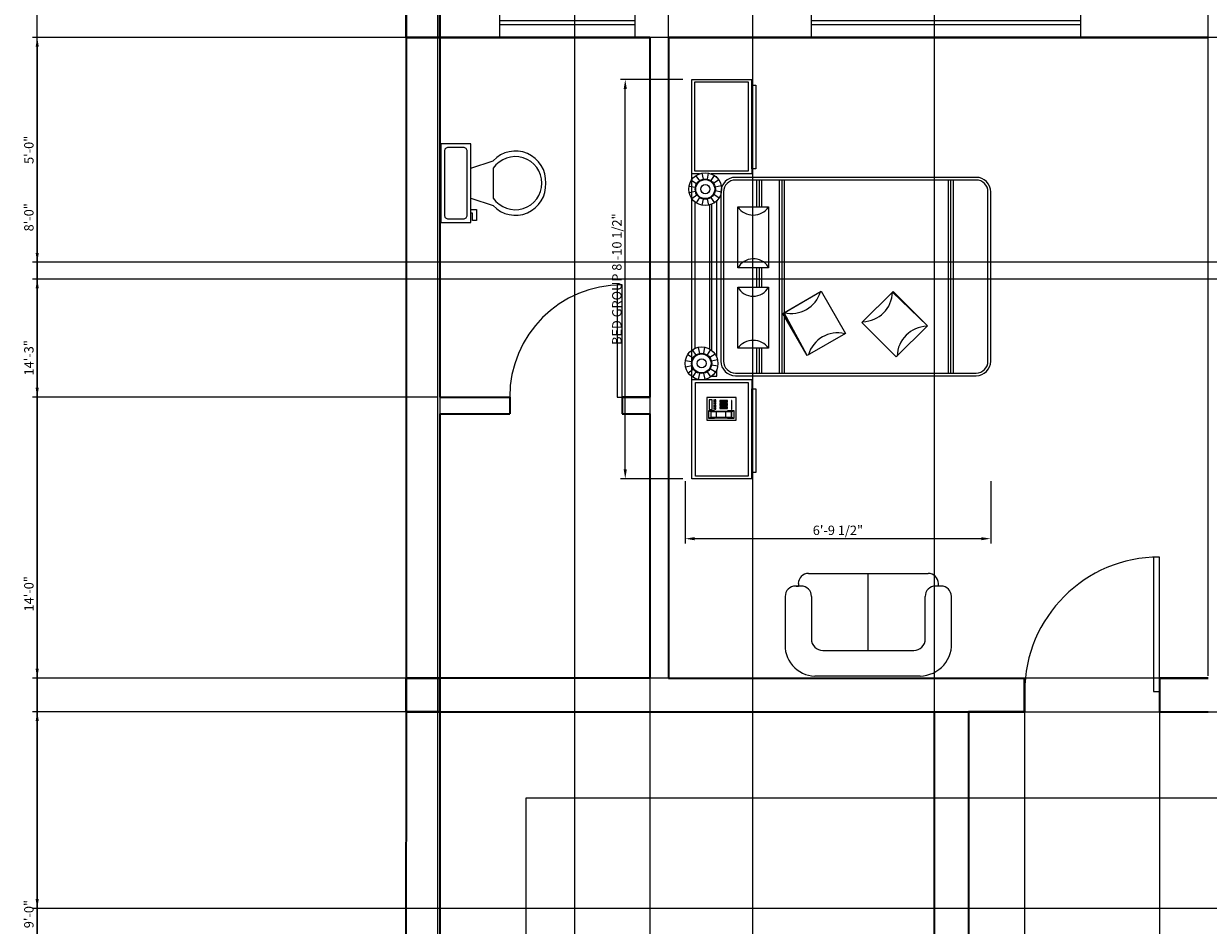
# Model space of a CAD drawing. Units: inches. Extents: x 1624 to 3956, y 1589 to 5028.
# Tile 9 of 16: x 1627 to 1943, y 2250 to 2490. Entities that reach past the tile are written whole.
import ezdxf

# ---------------------------------------------------------------- set-up
doc = ezdxf.new("R2010")
doc.units = ezdxf.units.IN
for name, color, linetype, lineweight in [('A-ANNO-DIMS', 2, 'Continuous', 13), ('A-COLS', 1, 'Continuous', 40), ('A-DOOR', 3, 'Continuous', 18), ('A-FLOR-CASE', 32, 'Continuous', 25), ('A-FLOR-FIXT', 9, 'Continuous', 18), ('A-FURN', 8, 'Continuous', 18), ('A-GLAZ', 4, 'Continuous', 18), ('A-WALL', 7, 'Continuous', 35)]:
    doc.layers.add(name, color=color, linetype=linetype, lineweight=lineweight)
doc.styles.get("Standard").update_dxf_attribs({"font": 'arial.ttf'})
doc.dimstyles.new('Copy of ISO-25', dxfattribs={"dimtxt": 2.5, "dimasz": 2.5, "dimexe": 1.25, "dimexo": 0.625, "dimtad": 1, "dimdec": 1, "dimlunit": 4, "dimtxsty": 'Standard', "dimcen": 2.5, "dimadec": 0, "dimazin": 0, "dimtfac": 1, "dimtdec": 1, "dimtmove": 0, "dimatfit": 3, "dimfxl": 1, "dimarcsym": 0})

# ---------------------------------------------------------------- blocks, each defined once
blk = doc.blocks.new('*U4')
for p, q in [((0, 0), (0, -6)), ((-40, 0), (-40, -6))]:
    blk.add_line(p, q)
blk.add_lwpolyline([(0, 0), (0, 40), (-1.75, 40), (-1.75, 0)], close=True)
blk.add_arc((0, 0), 40, 90, 180)
blk = doc.blocks.new('A$C18EB7ED0')
for p, q in [((0, 2.1539), (2.8801, 2.1539)), ((0, 1.7209), (0, 2.1539)), ((0.7156, 2.1539), (0.7156, 1.7209)), ((0.7332, 2.1483), (0.7713, 2.1237)), ((0.7653, 2.1814), (0.7911, 2.1442)), ((0.8076, 2.1998), (0.8172, 2.1555)), ((0.8537, 2.2006), (0.8456, 2.1559)), ((0.8966, 2.1836), (0.8721, 2.1455)), ((0.9298, 2.1515), (0.8925, 2.1257)), ((2.022, 2.155), (2.0478, 2.1177)), ((2.0643, 2.1733), (2.0739, 2.129)), ((2.1105, 2.1741), (2.1024, 2.1295)), ((2.1534, 2.1571), (2.1288, 2.119)), ((2.1997, 2.1), (2.1997, 2.1539)), ((2.8801, 2.1539), (2.8801, 1.7209)), ((0.0187, 2.129), (0.695, 2.129)), ((0.0187, 1.7489), (0.0187, 2.129)), ((0.695, 2.129), (0.695, 1.7489)), ((0.7162, 2.1054), (0.7608, 2.0973)), ((0.717, 2.0593), (0.7613, 2.0688)), ((0.9481, 2.1092), (0.9038, 2.0996)), ((0.9489, 2.0631), (0.9043, 2.0712)), ((0.941, 2.1314), (1.9968, 2.1314)), ((1.973, 2.0789), (2.0176, 2.0708)), ((1.9899, 2.1218), (2.028, 2.0973)), ((2.1865, 2.1251), (2.1493, 2.0992)), ((2.2049, 2.0827), (2.1606, 2.0731)), ((2.2184, 2.1337), (2.8624, 2.1337)), ((2.2184, 1.7489), (2.2184, 2.1337)), ((2.8624, 2.1337), (2.8624, 1.7489)), ((0.5857, 2.0461), (0.4227, 2.0461)), ((0.4227, 2.0461), (0.4227, 1.8353)), ((0.4366, 2.0335), (0.4439, 2.018)), ((0.4903, 2.0335), (0.4366, 2.0335)), ((0.4366, 2.0335), (0.4366, 1.9902)), ((0.4366, 1.9902), (0.4391, 1.9789)), ((0.4391, 1.9789), (0.4391, 1.9067)), ((0.4824, 2.018), (0.4439, 2.018)), ((0.4824, 2.018), (0.4439, 2.018)), ((0.4439, 2.018), (0.4439, 1.8697)), ((0.4824, 1.978), (0.4439, 1.978)), ((0.4824, 2.018), (0.4903, 2.0335)), ((0.4824, 1.8697), (0.4824, 2.018)), ((0.4903, 1.9902), (0.4871, 1.9789)), ((0.4871, 1.9789), (0.4871, 1.908)), ((0.4903, 1.9902), (0.4903, 2.0338)), ((0.5706, 2.0307), (0.4996, 2.0307)), ((0.4996, 2.0307), (0.4996, 2.0082)), ((0.4996, 2.0082), (0.5706, 2.0082)), ((0.514, 1.9963), (0.5013, 1.9963)), ((0.5013, 1.9963), (0.5013, 1.992)), ((0.5013, 1.992), (0.514, 1.992)), ((0.514, 1.9864), (0.5013, 1.9864)), ((0.5013, 1.9864), (0.5013, 1.9821)), ((0.5013, 1.9821), (0.514, 1.9821)), ((0.514, 1.992), (0.514, 1.9963)), ((0.514, 1.9821), (0.514, 1.9864)), ((0.5324, 1.9963), (0.5196, 1.9963)), ((0.5196, 1.9963), (0.5196, 1.992)), ((0.5196, 1.992), (0.5324, 1.992)), ((0.5324, 1.9864), (0.5196, 1.9864)), ((0.5196, 1.9864), (0.5196, 1.9821)), ((0.5196, 1.9821), (0.5324, 1.9821)), ((0.5324, 1.992), (0.5324, 1.9963)), ((0.5324, 1.9821), (0.5324, 1.9864)), ((0.5507, 1.9963), (0.538, 1.9963)), ((0.538, 1.9963), (0.538, 1.992)), ((0.538, 1.992), (0.5507, 1.992)), ((0.5507, 1.9864), (0.538, 1.9864)), ((0.538, 1.9864), (0.538, 1.9821)), ((0.538, 1.9821), (0.5507, 1.9821)), ((0.5507, 1.992), (0.5507, 1.9963)), ((0.5507, 1.9821), (0.5507, 1.9864)), ((0.5691, 1.9963), (0.5564, 1.9963)), ((0.5564, 1.9963), (0.5564, 1.992)), ((0.5564, 1.992), (0.5691, 1.992)), ((0.5691, 1.9864), (0.5564, 1.9864)), ((0.5564, 1.9864), (0.5564, 1.9821)), ((0.5564, 1.9821), (0.5691, 1.9821)), ((0.5691, 1.992), (0.5691, 1.9963)), ((0.5691, 1.9821), (0.5691, 1.9864)), ((0.5706, 2.0082), (0.5706, 2.0307)), ((0.5857, 1.8353), (0.5857, 2.0461)), ((0.7353, 2.0169), (0.7726, 2.0427)), ((0.7411, 2.0132), (0.7411, 1.9754)), ((0.7411, 1.9754), (0.7863, 1.9754)), ((0.7685, 1.9849), (0.7931, 2.023)), ((0.8114, 1.9679), (0.8195, 2.0125)), ((0.8575, 1.9687), (0.848, 2.013)), ((0.8999, 1.987), (0.8741, 2.0243)), ((0.8788, 1.9754), (2.0045, 1.9754)), ((0.9319, 2.0202), (0.8938, 2.0447)), ((1.9798, 2.0132), (0.9271, 2.0132)), ((1.9752, 2.0268), (0.9359, 2.0268)), ((1.9737, 2.0328), (2.0181, 2.0424)), ((1.9921, 1.9905), (2.0294, 2.0163)), ((2.0252, 1.9584), (2.0498, 1.9965)), ((2.0682, 1.9414), (2.0763, 1.986)), ((2.1143, 1.9422), (2.1047, 1.9865)), ((2.1566, 1.9605), (2.1308, 1.9978)), ((2.1887, 1.9937), (2.1506, 2.0183)), ((2.2056, 2.0366), (2.161, 2.0447)), ((2.1742, 1.9754), (2.1771, 1.9754)), ((2.1771, 1.9754), (2.1771, 1.9785)), ((2.1997, 1.7209), (2.1997, 2.0155)), ((0.4391, 1.9067), (0.4366, 1.8971)), ((0.4366, 1.8971), (0.4366, 1.8504)), ((0.4439, 1.9101), (0.4824, 1.9101)), ((0.4871, 1.908), (0.4903, 1.8971)), ((0.4903, 1.8499), (0.4903, 1.8971)), ((0.52, 1.9534), (0.5062, 1.9534)), ((0.5062, 1.9534), (0.5062, 1.9417)), ((0.5062, 1.9417), (0.52, 1.9417)), ((0.52, 1.9385), (0.5062, 1.9385)), ((0.5062, 1.9385), (0.5062, 1.9269)), ((0.5062, 1.9269), (0.52, 1.9269)), ((0.52, 1.9237), (0.5062, 1.9237)), ((0.5062, 1.9237), (0.5062, 1.9121)), ((0.5062, 1.9121), (0.52, 1.9121)), ((0.52, 1.9089), (0.5062, 1.9089)), ((0.5062, 1.9089), (0.5062, 1.8972)), ((0.5062, 1.8972), (0.52, 1.8972)), ((0.52, 1.9417), (0.52, 1.9534)), ((0.52, 1.9269), (0.52, 1.9385)), ((0.52, 1.9121), (0.52, 1.9237)), ((0.52, 1.8972), (0.52, 1.9089)), ((0.5426, 1.9534), (0.5288, 1.9534)), ((0.5288, 1.9534), (0.5288, 1.9417)), ((0.5288, 1.9417), (0.5426, 1.9417)), ((0.5426, 1.9385), (0.5288, 1.9385)), ((0.5288, 1.9385), (0.5288, 1.9269)), ((0.5288, 1.9269), (0.5426, 1.9269)), ((0.5426, 1.9237), (0.5288, 1.9237)), ((0.5288, 1.9237), (0.5288, 1.9121)), ((0.5288, 1.9121), (0.5426, 1.9121)), ((0.5426, 1.9089), (0.5288, 1.9089)), ((0.5288, 1.9089), (0.5288, 1.8972)), ((0.5288, 1.8972), (0.5426, 1.8972)), ((0.5426, 1.9417), (0.5426, 1.9534)), ((0.5426, 1.9269), (0.5426, 1.9385)), ((0.5426, 1.9121), (0.5426, 1.9237)), ((0.5426, 1.8972), (0.5426, 1.9089)), ((0.5659, 1.9534), (0.5521, 1.9534)), ((0.5521, 1.9534), (0.5521, 1.9417)), ((0.5521, 1.9417), (0.5659, 1.9417)), ((0.5659, 1.9385), (0.5521, 1.9385)), ((0.5521, 1.9385), (0.5521, 1.9269)), ((0.5521, 1.9269), (0.5659, 1.9269)), ((0.5659, 1.9237), (0.5521, 1.9237)), ((0.5521, 1.9237), (0.5521, 1.9121)), ((0.5521, 1.9121), (0.5659, 1.9121)), ((0.5659, 1.9089), (0.5521, 1.9089)), ((0.5521, 1.9089), (0.5521, 1.8972)), ((0.5521, 1.8972), (0.5659, 1.8972)), ((0.5659, 1.9417), (0.5659, 1.9534)), ((0.5659, 1.9269), (0.5659, 1.9385)), ((0.5659, 1.9121), (0.5659, 1.9237)), ((0.5659, 1.8972), (0.5659, 1.9089)), ((2.0691, 1.9452), (0.8491, 1.9452)), ((2.0691, 1.926), (0.8491, 1.926)), ((0.4227, 1.8353), (0.5857, 1.8353)), ((0.4439, 1.8697), (0.4366, 1.8504)), ((0.4366, 1.8504), (0.4903, 1.8504)), ((0.4824, 1.8697), (0.4439, 1.8697)), ((0.4439, 1.8697), (0.4824, 1.8697)), ((0.4903, 1.8504), (0.4824, 1.8697)), ((0.5208, 1.8697), (0.5009, 1.8697)), ((0.5009, 1.8697), (0.5009, 1.8657)), ((0.5009, 1.8657), (0.5208, 1.8657)), ((0.5208, 1.8657), (0.5208, 1.8697)), ((0.5433, 1.8697), (0.5234, 1.8697)), ((0.5234, 1.8697), (0.5234, 1.8657)), ((0.5234, 1.8657), (0.5433, 1.8657)), ((0.5433, 1.8657), (0.5433, 1.8697)), ((0.5658, 1.8697), (0.546, 1.8697)), ((0.546, 1.8697), (0.546, 1.8657)), ((0.546, 1.8657), (0.5658, 1.8657)), ((0.5658, 1.8657), (0.5658, 1.8697)), ((0.7439, 1.8401), (0.7439, 0.1052)), ((0.7632, 1.8401), (0.7632, 0.1052)), ((0.9429, 1.8231), (1.3829, 1.8231)), ((0.9429, 1.601), (0.9429, 1.8231)), ((1.3829, 1.8231), (1.3829, 1.601)), ((1.5207, 1.601), (1.5207, 1.8231)), ((1.5207, 1.8231), (1.9608, 1.8231)), ((1.9608, 1.8231), (1.9608, 1.601)), ((2.155, 0.1052), (2.155, 1.8401)), ((2.1743, 0.1052), (2.1743, 1.8401)), ((0.7156, 1.7209), (0, 1.7209)), ((0, 1.7209), (0.6483, 1.7209)), ((0.695, 1.7489), (0.0187, 1.7489)), ((0.0462, 1.6929), (0.0462, 1.7209)), ((0.6483, 1.7209), (0.6483, 1.6929)), ((2.8801, 1.7209), (2.1997, 1.7209)), ((2.8624, 1.7489), (2.2184, 1.7489)), ((2.2369, 1.7209), (2.8801, 1.7209)), ((2.2369, 1.6929), (2.2369, 1.7209)), ((2.839, 1.7209), (2.839, 1.6929)), ((0.6483, 1.6929), (0.0462, 1.6929)), ((0.7632, 1.6858), (0.9429, 1.6858)), ((0.7632, 1.6678), (0.9429, 1.6678)), ((0.7632, 1.6498), (0.9429, 1.6498)), ((1.3829, 1.6858), (1.5207, 1.6858)), ((1.3829, 1.6678), (1.5207, 1.6678)), ((1.3829, 1.6498), (1.5207, 1.6498)), ((1.9608, 1.6858), (2.155, 1.6858)), ((1.9608, 1.6678), (2.155, 1.6678)), ((1.9608, 1.6498), (2.155, 1.6498)), ((2.839, 1.6929), (2.2369, 1.6929)), ((1.3829, 1.601), (0.9429, 1.601)), ((1.9608, 1.601), (1.5207, 1.601)), ((0.7632, 1.5215), (2.155, 1.5215)), ((0.7632, 1.5035), (2.155, 1.5035)), ((0.7632, 1.4855), (2.155, 1.4855)), ((0.8904, 1.3226), (1.1935, 1.4976)), ((0.8904, 1.3226), (1.1982, 1.4894)), ((1.1935, 1.4976), (1.3524, 1.2224)), ((1.1982, 1.4894), (1.3524, 1.2224)), ((1.0493, 1.0474), (0.8904, 1.3226)), ((1.0493, 1.0474), (0.8904, 1.3226)), ((1.3524, 1.2224), (1.0493, 1.0474)), ((1.3524, 1.2224), (1.0493, 1.0474)), ((0.8789, 0.6811), (1.1264, 0.9286)), ((0.8789, 0.6811), (1.1264, 0.9286)), ((1.1264, 0.9286), (1.3473, 0.7077)), ((1.1264, 0.9286), (1.3511, 0.7039)), ((1.3473, 0.7077), (1.1036, 0.4564)), ((1.3511, 0.7039), (1.1036, 0.4564)), ((1.1036, 0.4564), (0.8789, 0.6811)), ((1.1036, 0.4564), (0.8789, 0.6811)), ((0.7632, 0.3045), (2.155, 0.3045)), ((0.7632, 0.2865), (2.155, 0.2865)), ((0.7632, 0.2685), (2.155, 0.2685)), ((0.8491, 0.0193), (2.0691, 0.0193)), ((0.8491, 0), (2.0691, 0))]:
    blk.add_line(p, q)
for centre, radius in [((0.8326, 2.0842), 0.1182), ((0.8326, 2.0842), 0.0729), ((0.8326, 2.0842), 0.0684), ((2.0893, 2.0578), 0.1182), ((0.8326, 2.0842), 0.0328), ((2.0893, 2.0578), 0.0729), ((2.0893, 2.0578), 0.0684), ((2.0893, 2.0578), 0.0328)]:
    blk.add_circle(centre, radius)
for centre, radius, start, end in [((0.8491, 1.8401), 0.1052, 90, 180), ((0.8491, 1.8401), 0.0859, 90, 180), ((2.0691, 1.8401), 0.1052, 0, 90), ((2.0691, 1.8401), 0.0859, 0, 90), ((0.8604, 1.712), 0.1383, 306.59595, 53.40405), ((1.4431, 1.712), 0.1263, 118.46186, 241.53814), ((1.4584, 1.7106), 0.1286, 303.40233, 61.02638), ((2.0371, 1.712), 0.1347, 124.50267, 235.49733), ((1.4126, 1.4383), 0.2204, 166.58792, 253.41208), ((0.8322, 1.1031), 0.2204, 346.58792, 73.41208), ((1.3534, 0.928), 0.2204, 181.58792, 268.41208), ((0.8795, 0.4541), 0.2204, 1.58792, 88.41208), ((0.8491, 0.1052), 0.1052, 180, 270), ((0.8491, 0.1052), 0.0859, 180, 270), ((2.0691, 0.1052), 0.1052, 270, 0), ((2.0691, 0.1052), 0.0859, 270, 0)]:
    blk.add_arc(centre, radius, start, end)
blk = doc.blocks.new('*U14')
for p, q in [((241.3, -152.4), (241.3, -50.8)), ((-254, -215.9), (-203.2, -215.9)), ((-254, -241.3), (-254, -215.9)), ((-203.2, -215.9), (-203.2, -203.2)), ((-177.8, -203.2), (-177.8, -241.3)), ((-101.6, -203.2), (-152.4, -355.6)), ((101.6, -203.2), (152.4, -355.6)), ((-177.8, -241.3), (-254, -241.3)), ((101.6, -355.6), (-101.6, -355.6))]:
    blk.add_line(p, q)
blk.add_lwpolyline([(266.7, -203.2), (266.7, 0), (-266.7, 0), (-266.7, -203.2)], close=True)
for points in [[(-241.3, -50.8), (-241.3, -152.4)], [(215.9, -25.4), (-215.9, -25.4)], [(-215.9, -177.8), (215.9, -177.8)]]:
    blk.add_lwpolyline(points)
for centre, radius, start, end in [((-219.075, -47.625), 22.45064, 81.8699, 188.1301), ((219.075, -47.625), 22.45064, 351.8699, 98.1301), ((-219.075, -155.575), 22.45064, 171.869898, 278.1301), ((219.075, -155.575), 22.45064, 261.8699, 8.1301), ((-12.12088, -505.93752), 205.61935, 133.01722, 273.38), ((0.94996, -504.77674), 181.02486, 124.50543, 269.7), ((-0.94742, -504.77674), 181.02486, 270.3, 55.4946), ((12.12342, -505.93752), 205.61935, 266.62, 46.9828)]:
    blk.add_arc(centre, radius, start, end)
blk = doc.blocks.new('A$C6D011943')
for p, q in [((1.448, 1.089), (0.332, 1.089)), ((1.364, 0.818), (0.398, 0.818)), ((0.881, 0.818), (0.881, 0)), ((0, 0.709), (0, 0.247)), ((0.278, 0.697), (0.278, 0.244)), ((1.485, 0.244), (1.485, 0.697)), ((1.762, 0.247), (1.762, 0.727)), ((0.109, 0.136), (0.169, 0.136)), ((0.139, 0.109), (0.139, 0.136)), ((1.593, 0.136), (1.654, 0.136)), ((1.648, 0.136), (1.623, 0.136)), ((1.623, 0.109), (1.623, 0.136)), ((1.515, 0), (0.247, 0))]:
    blk.add_line(p, q)
for centre, radius, start, end in [((0.339, 0.748), 0.342, 91.2564, 186.501), ((1.441, 0.766), 0.324, 353.159, 88.6697), ((0.398, 0.697), 0.121, 90, 180), ((1.364, 0.697), 0.121, 0, 90), ((0.109, 0.244), 0.109, 180, 270), ((0.169, 0.244), 0.109, 270, 0), ((1.593, 0.244), 0.109, 180, 270), ((1.654, 0.244), 0.109, 270, 0), ((0.247, 0.109), 0.109, 180, 270), ((1.515, 0.109), 0.109, 270, 0)]:
    blk.add_arc(centre, radius, start, end)
blk = doc.blocks.new('COLUMN-9x9')
for p, q in [((0, 0), (0, 9)), ((0, 9), (9, 9)), ((9, 9), (9, 0)), ((9, 0), (0, 0))]:
    blk.add_line(p, q)
blk = doc.blocks.new('WINDOW-36IN')
for p, q in [((0, 0), (0, 9)), ((36, 9), (36, 0)), ((0, 4.5), (36, 4.5)), ((0, 3.5), (36, 3.5))]:
    blk.add_line(p, q)
blk = doc.blocks.new('WINDOW-72IN')
for p, q in [((0, 9), (0, 0)), ((72, 0), (72, 9)), ((0, 4.5), (72, 4.5)), ((0, 3.5), (72, 3.5))]:
    blk.add_line(p, q)
blk = doc.blocks.new('*D60')
at = {"layer": 'A-ANNO-DIMS', "color": 0, "lineweight": -2, "transparency": 16777216}
for p, q in [((1802.37, 2475.57), (1785.76, 2475.57)), ((1787.01, 2371.48), (1787.01, 2473.07)), ((1802.37, 2368.98), (1785.76, 2368.98))]:
    blk.add_line(p, q, dxfattribs=at)
at = {"layer": 'A-ANNO-DIMS', "color": 0, "transparency": 16777216}
for points in [[(1786.59, 2473.07), (1787.42, 2473.07), (1787.01, 2475.57)], [(1786.59, 2371.48), (1787.42, 2371.48), (1787.01, 2368.98)]]:
    blk.add_solid(points, dxfattribs=at)
at = {"layer": 'Defpoints', "color": 0, "transparency": 16777216}
for p in [(1787.01, 2475.57), (1803, 2475.57), (1803, 2368.98)]:
    blk.add_point(p, dxfattribs=at)
at = {"layer": 'A-ANNO-DIMS', "color": 0, "transparency": 16777216, "insert": (1785.09, 2422.28), "char_height": 2.5, "attachment_point": 5, "rotation": 90}
blk.add_mtext('BED GROUP 8\'-10 1/2"', dxfattribs=at)
blk = doc.blocks.new('*D61')
at = {"layer": 'A-ANNO-DIMS', "color": 0, "lineweight": -2, "transparency": 16777216}
for p, q in [((1803, 2368.36), (1803, 2351.75)), ((1884.51, 2368.36), (1884.51, 2351.75)), ((1882.01, 2353), (1805.5, 2353))]:
    blk.add_line(p, q, dxfattribs=at)
at = {"layer": 'A-ANNO-DIMS', "color": 0, "transparency": 16777216}
for points in [[(1805.5, 2353.41), (1805.5, 2352.58), (1803, 2353)], [(1882.01, 2353.41), (1882.01, 2352.58), (1884.51, 2353)]]:
    blk.add_solid(points, dxfattribs=at)
at = {"layer": 'Defpoints', "color": 0, "transparency": 16777216}
for p in [(1803, 2368.98), (1884.51, 2368.98), (1803, 2353)]:
    blk.add_point(p, dxfattribs=at)
at = {"layer": 'A-ANNO-DIMS', "color": 0, "transparency": 16777216, "insert": (1843.75, 2354.91), "char_height": 2.5, "attachment_point": 5}
blk.add_mtext('6\'-9 1/2"', dxfattribs=at)
blk = doc.blocks.new('*D69')
at = {"layer": 'A-ANNO-DIMS', "color": 0, "lineweight": -2, "transparency": 16777216}
for p, q in [((1727.95, 2495.79), (1628.86, 2495.79)), ((1630.11, 1775.29), (1630.11, 2493.29)), ((1726.95, 1772.79), (1628.86, 1772.79))]:
    blk.add_line(p, q, dxfattribs=at)
at = {"layer": 'A-ANNO-DIMS', "color": 0, "transparency": 16777216}
for points in [[(1629.69, 2493.29), (1630.53, 2493.29), (1630.11, 2495.79)], [(1629.69, 1775.29), (1630.53, 1775.29), (1630.11, 1772.79)]]:
    blk.add_solid(points, dxfattribs=at)
at = {"layer": 'Defpoints', "color": 0, "transparency": 16777216}
for p in [(1630.11, 2495.79), (1728.58, 2495.79), (1727.58, 1772.79)]:
    blk.add_point(p, dxfattribs=at)
at = {"layer": 'A-ANNO-DIMS', "color": 0, "transparency": 16777216, "insert": (1628.21, 2134.29), "char_height": 2.5, "attachment_point": 5, "rotation": 90}
blk.add_mtext('60\'-3"', dxfattribs=at)
blk = doc.blocks.new('*D75')
at = {"layer": 'A-ANNO-DIMS', "color": 0, "lineweight": -2, "transparency": 16777216}
for p, q in [((1737.58, 2486.17), (1737.58, 1589.9)), ((1793.58, 2486.17), (1793.58, 1589.9)), ((1740.08, 1591.15), (1791.08, 1591.15))]:
    blk.add_line(p, q, dxfattribs=at)
at = {"layer": 'A-ANNO-DIMS', "color": 0, "transparency": 16777216}
for points in [[(1740.08, 1591.57), (1740.08, 1590.73), (1737.58, 1591.15)], [(1791.08, 1591.57), (1791.08, 1590.73), (1793.58, 1591.15)]]:
    blk.add_solid(points, dxfattribs=at)
at = {"layer": 'Defpoints', "color": 0, "transparency": 16777216}
for p in [(1737.58, 2486.79), (1793.58, 2486.79), (1793.58, 1591.15)]:
    blk.add_point(p, dxfattribs=at)
at = {"layer": 'A-ANNO-DIMS', "color": 0, "transparency": 16777216, "insert": (1765.58, 1593.05), "char_height": 2.5, "attachment_point": 5}
blk.add_mtext('4\'-8"', dxfattribs=at)
blk = doc.blocks.new('*D76')
at = {"layer": 'A-ANNO-DIMS', "color": 0, "lineweight": -2, "transparency": 16777216}
for p, q in [((1736.95, 2486.79), (1628.86, 2486.79)), ((1630.11, 2484.29), (1630.11, 2393.29)), ((1736.95, 2390.79), (1628.86, 2390.79))]:
    blk.add_line(p, q, dxfattribs=at)
at = {"layer": 'A-ANNO-DIMS', "color": 0, "transparency": 16777216}
for points in [[(1629.69, 2484.29), (1630.53, 2484.29), (1630.11, 2486.79)], [(1629.69, 2393.29), (1630.53, 2393.29), (1630.11, 2390.79)]]:
    blk.add_solid(points, dxfattribs=at)
at = {"layer": 'Defpoints', "color": 0, "transparency": 16777216}
for p in [(1737.58, 2486.79), (1630.11, 2390.79), (1737.58, 2390.79)]:
    blk.add_point(p, dxfattribs=at)
at = {"layer": 'A-ANNO-DIMS', "color": 0, "transparency": 16777216, "insert": (1628.21, 2438.79), "char_height": 2.5, "attachment_point": 5, "rotation": 90}
blk.add_mtext('8\'-0"', dxfattribs=at)
blk = doc.blocks.new('*D77')
at = {"layer": 'A-ANNO-DIMS', "color": 0, "lineweight": -2, "transparency": 16777216}
for p, q in [((1798.58, 2316.42), (1798.58, 2612.84)), ((1801.08, 2611.59), (1940.08, 2611.59)), ((1942.58, 2316.42), (1942.58, 2612.84))]:
    blk.add_line(p, q, dxfattribs=at)
at = {"layer": 'A-ANNO-DIMS', "color": 0, "transparency": 16777216}
for points in [[(1801.08, 2612.01), (1801.08, 2611.18), (1798.58, 2611.59)], [(1940.08, 2612.01), (1940.08, 2611.18), (1942.58, 2611.59)]]:
    blk.add_solid(points, dxfattribs=at)
at = {"layer": 'Defpoints', "color": 0, "transparency": 16777216}
for p in [(1942.58, 2611.59), (1798.58, 2315.79), (1942.58, 2315.79)]:
    blk.add_point(p, dxfattribs=at)
at = {"layer": 'A-ANNO-DIMS', "color": 0, "transparency": 16777216, "insert": (1870.58, 2613.5), "char_height": 2.5, "attachment_point": 5}
blk.add_mtext('12\'-0"', dxfattribs=at)
blk = doc.blocks.new('*D78')
at = {"layer": 'A-ANNO-DIMS', "color": 0, "lineweight": -2, "transparency": 16777216}
for p, q in [((1941.95, 2486.79), (1628.86, 2486.79)), ((1630.11, 2484.29), (1630.11, 2318.29)), ((1941.95, 2315.79), (1628.86, 2315.79))]:
    blk.add_line(p, q, dxfattribs=at)
at = {"layer": 'A-ANNO-DIMS', "color": 0, "transparency": 16777216}
for points in [[(1629.69, 2484.29), (1630.53, 2484.29), (1630.11, 2486.79)], [(1629.69, 2318.29), (1630.53, 2318.29), (1630.11, 2315.79)]]:
    blk.add_solid(points, dxfattribs=at)
at = {"layer": 'Defpoints', "color": 0, "transparency": 16777216}
for p in [(1942.58, 2486.79), (1630.11, 2315.79), (1942.58, 2315.79)]:
    blk.add_point(p, dxfattribs=at)
at = {"layer": 'A-ANNO-DIMS', "color": 0, "transparency": 16777216, "insert": (1628.21, 2401.29), "char_height": 2.5, "attachment_point": 5, "rotation": 90}
blk.add_mtext('14\'-3"', dxfattribs=at)
blk = doc.blocks.new('*D79')
at = {"layer": 'A-ANNO-DIMS', "color": 0, "lineweight": -2, "transparency": 16777216}
for p, q in [((2090.95, 2422.29), (1628.86, 2422.29)), ((1630.11, 2419.79), (1630.11, 2256.79)), ((2090.95, 2254.29), (1628.86, 2254.29))]:
    blk.add_line(p, q, dxfattribs=at)
at = {"layer": 'A-ANNO-DIMS', "color": 0, "transparency": 16777216}
for points in [[(1629.69, 2419.79), (1630.53, 2419.79), (1630.11, 2422.29)], [(1629.69, 2256.79), (1630.53, 2256.79), (1630.11, 2254.29)]]:
    blk.add_solid(points, dxfattribs=at)
at = {"layer": 'Defpoints', "color": 0, "transparency": 16777216}
for p in [(2091.58, 2422.29), (1630.11, 2254.29), (2091.58, 2254.29)]:
    blk.add_point(p, dxfattribs=at)
at = {"layer": 'A-ANNO-DIMS', "color": 0, "transparency": 16777216, "insert": (1628.21, 2338.29), "char_height": 2.5, "attachment_point": 5, "rotation": 90}
blk.add_mtext('14\'-0"', dxfattribs=at)
blk = doc.blocks.new('*D82')
at = {"layer": 'A-ANNO-DIMS', "color": 0, "lineweight": -2, "transparency": 16777216}
for p, q in [((1737.58, 2306.17), (1737.58, 1589.9)), ((1869.56, 2306.17), (1869.56, 1589.9)), ((1740.08, 1591.15), (1867.06, 1591.15))]:
    blk.add_line(p, q, dxfattribs=at)
at = {"layer": 'A-ANNO-DIMS', "color": 0, "transparency": 16777216}
for points in [[(1740.08, 1591.57), (1740.08, 1590.73), (1737.58, 1591.15)], [(1867.06, 1591.57), (1867.06, 1590.73), (1869.56, 1591.15)]]:
    blk.add_solid(points, dxfattribs=at)
at = {"layer": 'Defpoints', "color": 0, "transparency": 16777216}
for p in [(1737.58, 2306.79), (1869.56, 2306.79), (1869.56, 1591.15)]:
    blk.add_point(p, dxfattribs=at)
at = {"layer": 'A-ANNO-DIMS', "color": 0, "transparency": 16777216, "insert": (1803.57, 1593.05), "char_height": 2.5, "attachment_point": 5}
blk.add_mtext('11\'-0"', dxfattribs=at)
blk = doc.blocks.new('*D83')
at = {"layer": 'A-ANNO-DIMS', "color": 0, "lineweight": -2, "transparency": 16777216}
for p, q in [((1868.93, 2306.79), (1628.86, 2306.79)), ((1630.11, 2304.29), (1630.11, 2201.29)), ((1868.93, 2198.79), (1628.86, 2198.79))]:
    blk.add_line(p, q, dxfattribs=at)
at = {"layer": 'A-ANNO-DIMS', "color": 0, "transparency": 16777216}
for points in [[(1629.69, 2304.29), (1630.53, 2304.29), (1630.11, 2306.79)], [(1629.69, 2201.29), (1630.53, 2201.29), (1630.11, 2198.79)]]:
    blk.add_solid(points, dxfattribs=at)
at = {"layer": 'Defpoints', "color": 0, "transparency": 16777216}
for p in [(1869.56, 2306.79), (1630.11, 2198.79), (1869.56, 2198.79)]:
    blk.add_point(p, dxfattribs=at)
at = {"layer": 'A-ANNO-DIMS', "color": 0, "transparency": 16777216, "insert": (1628.21, 2252.79), "char_height": 2.5, "attachment_point": 5, "rotation": 90}
blk.add_mtext('9\'-0"', dxfattribs=at)
blk = doc.blocks.new('*D86')
at = {"layer": 'A-ANNO-DIMS', "color": 0, "lineweight": -2, "transparency": 16777216}
for p, q in [((1737.01, 1953.42), (1737.01, 2612.84)), ((1739.51, 2611.59), (1818.51, 2611.59)), ((1821.01, 1953.42), (1821.01, 2612.84))]:
    blk.add_line(p, q, dxfattribs=at)
at = {"layer": 'A-ANNO-DIMS', "color": 0, "transparency": 16777216}
for points in [[(1739.51, 2612.01), (1739.51, 2611.18), (1737.01, 2611.59)], [(1818.51, 2612.01), (1818.51, 2611.18), (1821.01, 2611.59)]]:
    blk.add_solid(points, dxfattribs=at)
at = {"layer": 'Defpoints', "color": 0, "transparency": 16777216}
for p in [(1821.01, 2611.59), (1737.01, 1952.79), (1821.01, 1952.79)]:
    blk.add_point(p, dxfattribs=at)
at = {"layer": 'A-ANNO-DIMS', "color": 0, "transparency": 16777216, "insert": (1779.01, 2613.5), "char_height": 2.5, "attachment_point": 5}
blk.add_mtext('7\'-0"', dxfattribs=at)
blk = doc.blocks.new('*D89')
at = {"layer": 'A-ANNO-DIMS', "color": 0, "lineweight": -2, "transparency": 16777216}
for p, q in [((2090.95, 2486.79), (1628.86, 2486.79)), ((1630.11, 2484.29), (1630.11, 2429.29)), ((2090.95, 2426.79), (1628.86, 2426.79))]:
    blk.add_line(p, q, dxfattribs=at)
at = {"layer": 'A-ANNO-DIMS', "color": 0, "transparency": 16777216}
for points in [[(1629.69, 2484.29), (1630.53, 2484.29), (1630.11, 2486.79)], [(1629.69, 2429.29), (1630.53, 2429.29), (1630.11, 2426.79)]]:
    blk.add_solid(points, dxfattribs=at)
at = {"layer": 'Defpoints', "color": 0, "transparency": 16777216}
for p in [(2091.58, 2486.79), (1630.11, 2426.79), (2091.58, 2426.79)]:
    blk.add_point(p, dxfattribs=at)
at = {"layer": 'A-ANNO-DIMS', "color": 0, "transparency": 16777216, "insert": (1628.21, 2456.79), "char_height": 2.5, "attachment_point": 5, "rotation": 90}
blk.add_mtext('5\'-0"', dxfattribs=at)
blk = doc.blocks.new('*D94')
at = {"layer": 'A-ANNO-DIMS', "color": 0, "lineweight": -2, "transparency": 16777216}
for p, q in [((1893.52, 2315.17), (1893.52, 1589.9)), ((1929.52, 2315.17), (1929.52, 1589.9)), ((1896.02, 1591.15), (1927.02, 1591.15))]:
    blk.add_line(p, q, dxfattribs=at)
at = {"layer": 'A-ANNO-DIMS', "color": 0, "transparency": 16777216}
for points in [[(1896.02, 1591.57), (1896.02, 1590.73), (1893.52, 1591.15)], [(1927.02, 1591.57), (1927.02, 1590.73), (1929.52, 1591.15)]]:
    blk.add_solid(points, dxfattribs=at)
at = {"layer": 'Defpoints', "color": 0, "transparency": 16777216}
for p in [(1893.52, 2315.79), (1929.52, 2315.79), (1929.52, 1591.15)]:
    blk.add_point(p, dxfattribs=at)
at = {"layer": 'A-ANNO-DIMS', "color": 0, "transparency": 16777216, "insert": (1911.52, 1593.05), "char_height": 2.5, "attachment_point": 5}
blk.add_mtext('3\'-0"', dxfattribs=at)
blk = doc.blocks.new('*D97')
at = {"layer": 'A-ANNO-DIMS', "color": 0, "lineweight": -2, "transparency": 16777216}
for p, q in [((1773.53, 1773.42), (1773.53, 2612.84)), ((1776.03, 2611.59), (1867.03, 2611.59)), ((1869.53, 1773.42), (1869.53, 2612.84))]:
    blk.add_line(p, q, dxfattribs=at)
at = {"layer": 'A-ANNO-DIMS', "color": 0, "transparency": 16777216}
for points in [[(1776.03, 2612.01), (1776.03, 2611.18), (1773.53, 2611.59)], [(1867.03, 2612.01), (1867.03, 2611.18), (1869.53, 2611.59)]]:
    blk.add_solid(points, dxfattribs=at)
at = {"layer": 'Defpoints', "color": 0, "transparency": 16777216}
for p in [(1869.53, 2611.59), (1773.53, 1772.79), (1869.53, 1772.79)]:
    blk.add_point(p, dxfattribs=at)
at = {"layer": 'A-ANNO-DIMS', "color": 0, "transparency": 16777216, "insert": (1821.53, 2613.5), "char_height": 2.5, "attachment_point": 5}
blk.add_mtext('8\'-0"', dxfattribs=at)
blk = doc.blocks.new('*D100')
at = {"layer": 'A-ANNO-DIMS', "color": 0, "lineweight": -2, "transparency": 16777216}
for p, q in [((1738.2, 2306.79), (2217.63, 2306.79)), ((2216.38, 2286.28), (2216.38, 2304.29)), ((1761.2, 2283.78), (2217.63, 2283.78))]:
    blk.add_line(p, q, dxfattribs=at)
at = {"layer": 'A-ANNO-DIMS', "color": 0, "transparency": 16777216}
for points in [[(2215.96, 2304.29), (2216.8, 2304.29), (2216.38, 2306.79)], [(2215.96, 2286.28), (2216.8, 2286.28), (2216.38, 2283.78)]]:
    blk.add_solid(points, dxfattribs=at)
at = {"layer": 'Defpoints', "color": 0, "transparency": 16777216}
for p in [(1737.58, 2306.79), (2216.38, 2306.79), (1760.58, 2283.78)]:
    blk.add_point(p, dxfattribs=at)
at = {"layer": 'A-ANNO-DIMS', "color": 0, "transparency": 16777216, "insert": (2214.5, 2295.29), "char_height": 2.5, "attachment_point": 5, "rotation": 90}
blk.add_mtext('1\'-11"', dxfattribs=at)
blk = doc.blocks.new('*D101')
at = {"layer": 'A-ANNO-DIMS', "color": 0, "lineweight": -2, "transparency": 16777216}
for p, q in [((1737.01, 1782.42), (1737.01, 2612.84)), ((1739.51, 2611.59), (1771.03, 2611.59)), ((1773.53, 1782.42), (1773.53, 2612.84))]:
    blk.add_line(p, q, dxfattribs=at)
at = {"layer": 'A-ANNO-DIMS', "color": 0, "transparency": 16777216}
for points in [[(1739.51, 2612.01), (1739.51, 2611.18), (1737.01, 2611.59)], [(1771.03, 2612.01), (1771.03, 2611.18), (1773.53, 2611.59)]]:
    blk.add_solid(points, dxfattribs=at)
at = {"layer": 'Defpoints', "color": 0, "transparency": 16777216}
for p in [(1773.53, 2611.59), (1737.01, 1781.79), (1773.53, 1781.79)]:
    blk.add_point(p, dxfattribs=at)
at = {"layer": 'A-ANNO-DIMS', "color": 0, "transparency": 16777216, "insert": (1755.27, 2613.51), "char_height": 2.5, "attachment_point": 5}
blk.add_mtext('3\'-0 1/2"', dxfattribs=at)

msp = doc.modelspace()

# ---------------------------------------------------------------- linework, layer by layer
at = {"layer": 'A-FLOR-CASE'}
for p, q in [((1760.58, 2283.78), (1869.56, 2283.78)), ((1760.58, 2240.37), (1760.58, 2283.78))]:
    msp.add_line(p, q, dxfattribs=at)
at = {"layer": 'A-WALL'}
for p, q in [((1728.58, 2486.79), (1728.58, 2495.79)), ((1728.58, 2486.79), (1728.58, 2301.8)), ((1737.58, 2486.79), (1742.08, 2486.79)), ((1793.58, 2486.79), (1737.58, 2486.79)), ((1737.58, 2486.79), (1737.58, 2390.79)), ((1737.58, 2486.79), (1737.58, 2390.79)), ((1737.58, 2486.79), (1753.58, 2486.79)), ((1742.08, 2486.79), (1758.08, 2486.79)), ((1758.08, 2486.79), (1793.58, 2486.79)), ((1793.58, 2486.79), (1793.58, 2390.79)), ((1798.58, 2486.79), (1841.08, 2486.79)), ((1942.58, 2486.79), (1798.58, 2486.79)), ((1798.58, 2486.79), (1798.58, 2315.79)), ((1841.08, 2486.79), (1913.08, 2486.79)), ((1913.08, 2486.79), (1942.58, 2486.79)), ((1737.58, 2390.79), (1756.17, 2390.79)), ((1756.17, 2390.79), (1756.17, 2386.29)), ((1793.58, 2390.79), (1786.17, 2390.79)), ((1786.17, 2390.79), (1786.17, 2386.29)), ((1786.17, 2390.79), (1793.58, 2390.79)), ((1737.58, 2386.29), (1756.17, 2386.29)), ((1737.58, 2386.29), (1737.58, 2315.79)), ((1786.17, 2386.29), (1793.58, 2386.29)), ((1793.58, 2386.29), (1793.58, 2315.79)), ((1793.58, 2315.79), (1737.58, 2315.79)), ((1798.58, 2315.79), (1893.52, 2315.79)), ((1893.52, 2306.79), (1893.52, 2315.79)), ((1942.58, 2315.79), (1929.52, 2315.79)), ((1929.52, 2315.79), (1929.52, 2306.79)), ((1929.52, 2315.79), (1942.58, 2315.79)), ((1737.58, 2306.79), (1893.52, 2306.79)), ((1737.58, 2306.79), (1737.58, 2198.79)), ((1869.56, 2239.87), (1869.56, 2306.79)), ((1893.52, 2306.79), (1878.56, 2306.79)), ((1878.56, 2306.79), (1878.56, 2239.87)), ((1929.52, 2306.79), (1942.58, 2306.79)), ((1728.58, 2301.8), (1727.58, 1772.79))]:
    msp.add_line(p, q, dxfattribs=at)

# ---------------------------------------------------------------- block references
at = {"layer": 'A-COLS'}
msp.add_blockref('COLUMN-9x9', (1728.58, 2486.79), dxfattribs=at)
at = {"layer": 'A-COLS', "rotation": 180}
msp.add_blockref('COLUMN-9x9', (1737.58, 2315.79), dxfattribs=at)
at = {"layer": 'A-DOOR'}
for p, xscale, yscale, zscale in [((1786.17, 2390.79), 0.7497586430423404, 0.7497586430423404, 0.7497586430423404), ((1929.52, 2312.18), 0.8982084914173354, 0.8982084914173354, 0.8982084914173354)]:
    msp.add_blockref('*U4', p, dxfattribs=dict(at, xscale=xscale, yscale=yscale, zscale=zscale))
at = {"layer": 'A-FLOR-FIXT', "xscale": 0.0393700787401575, "yscale": 0.0393700787401575, "zscale": 0.0393700787401575, "rotation": 89.99999999999999}
msp.add_blockref('*U14', (1737.79, 2447.9), dxfattribs=at)
at = {"layer": 'A-FURN'}
for name, p, xscale, yscale, zscale, rotation in [('A$C18EB7ED0', (1884.51, 2368.98), 37.00871928414762, 37.00871928414762, 37.00871928414762, 90), ('A$C6D011943', (1874.02, 2343.74), 25.14761962403201, 25.14761962403201, 25.14761962403201, 180)]:
    msp.add_blockref(name, p, dxfattribs=dict(at, xscale=xscale, yscale=yscale, zscale=zscale, rotation=rotation))
at = {"layer": 'A-GLAZ'}
for name, p in [('WINDOW-36IN', (1753.58, 2486.79)), ('WINDOW-72IN', (1836.58, 2486.79))]:
    msp.add_blockref(name, p, dxfattribs=at)

# ---------------------------------------------------------------- dimensions: what is measured, and where the dimension line sits
at = {"layer": 'A-ANNO-DIMS'}
for base, p1, p2, picture, middle in [((1773.53, 2611.59), (1737.01, 1781.79), (1773.53, 1781.79), '*D101', (1755.27, 2613.51)), ((1821.01, 2611.59), (1737.01, 1952.79), (1821.01, 1952.79), '*D86', (1779.01, 2613.5)), ((1869.53, 2611.59), (1773.53, 1772.79), (1869.53, 1772.79), '*D97', (1821.53, 2613.5)), ((1942.58, 2611.59), (1798.58, 2315.79), (1942.58, 2315.79), '*D77', (1870.58, 2613.5)), ((1793.58, 1591.15), (1737.58, 2486.79), (1793.58, 2486.79), '*D75', (1765.58, 1593.05)), ((1929.52, 1591.15), (1893.52, 2315.79), (1929.52, 2315.79), '*D94', (1911.52, 1593.05)), ((1869.56, 1591.15), (1737.58, 2306.79), (1869.56, 2306.79), '*D82', (1803.57, 1593.05))]:
    dim = msp.add_linear_dim(base=base, p1=p1, p2=p2, dimstyle='Copy of ISO-25', override={"dimdec": 1, "dimlfac": 1, "dimrnd": 0, "dimzin": 1, "dimdsep": 46, "dimlunit": 4, "dimfrac": 2}, dxfattribs=at)
    dim.commit()
    dim.dimension.update_dxf_attribs({"geometry": picture, "text_midpoint": middle})
for base, p1, p2, angle, picture, middle in [((1630.11, 2495.79), (1727.58, 1772.79), (1728.58, 2495.79), 90, '*D69', (1628.21, 2134.29)), ((1630.11, 2390.79), (1737.58, 2486.79), (1737.58, 2390.79), 90, '*D76', (1628.21, 2438.79)), ((1630.11, 2315.79), (1942.58, 2486.79), (1942.58, 2315.79), 90, '*D78', (1628.21, 2401.29)), ((1630.11, 2426.79), (2091.58, 2486.79), (2091.58, 2426.79), 90, '*D89', (1628.21, 2456.79)), ((1630.11, 2254.29), (2091.58, 2422.29), (2091.58, 2254.29), 90, '*D79', (1628.21, 2338.29)), ((1803, 2353), (1884.51, 2368.98), (1803, 2368.98), 180, '*D61', (1843.75, 2354.91)), ((1630.11, 2198.79), (1869.56, 2306.79), (1869.56, 2198.79), 90, '*D83', (1628.21, 2252.79)), ((2216.38, 2306.79), (1760.58, 2283.78), (1737.58, 2306.79), 90, '*D100', (2214.5, 2295.29))]:
    dim = msp.add_linear_dim(base=base, p1=p1, p2=p2, angle=angle, dimstyle='Copy of ISO-25', override={"dimdec": 1, "dimlfac": 1, "dimrnd": 0, "dimzin": 1, "dimdsep": 46, "dimlunit": 4, "dimfrac": 2}, dxfattribs=at)
    dim.commit()
    dim.dimension.update_dxf_attribs({"geometry": picture, "text_midpoint": middle})
dim = msp.add_linear_dim(base=(1787.01, 2475.57), p1=(1803, 2368.98), p2=(1803, 2475.57), angle=90, text='BED GROUP <>', dimstyle='Copy of ISO-25', override={"dimdec": 1, "dimlfac": 1, "dimrnd": 0, "dimzin": 1, "dimdsep": 46, "dimlunit": 4, "dimfrac": 2}, dxfattribs=at)
dim.commit()
dim.dimension.update_dxf_attribs({"geometry": '*D60', "text_midpoint": (1785.09, 2422.28)})

doc.saveas('drawing.dxf')
